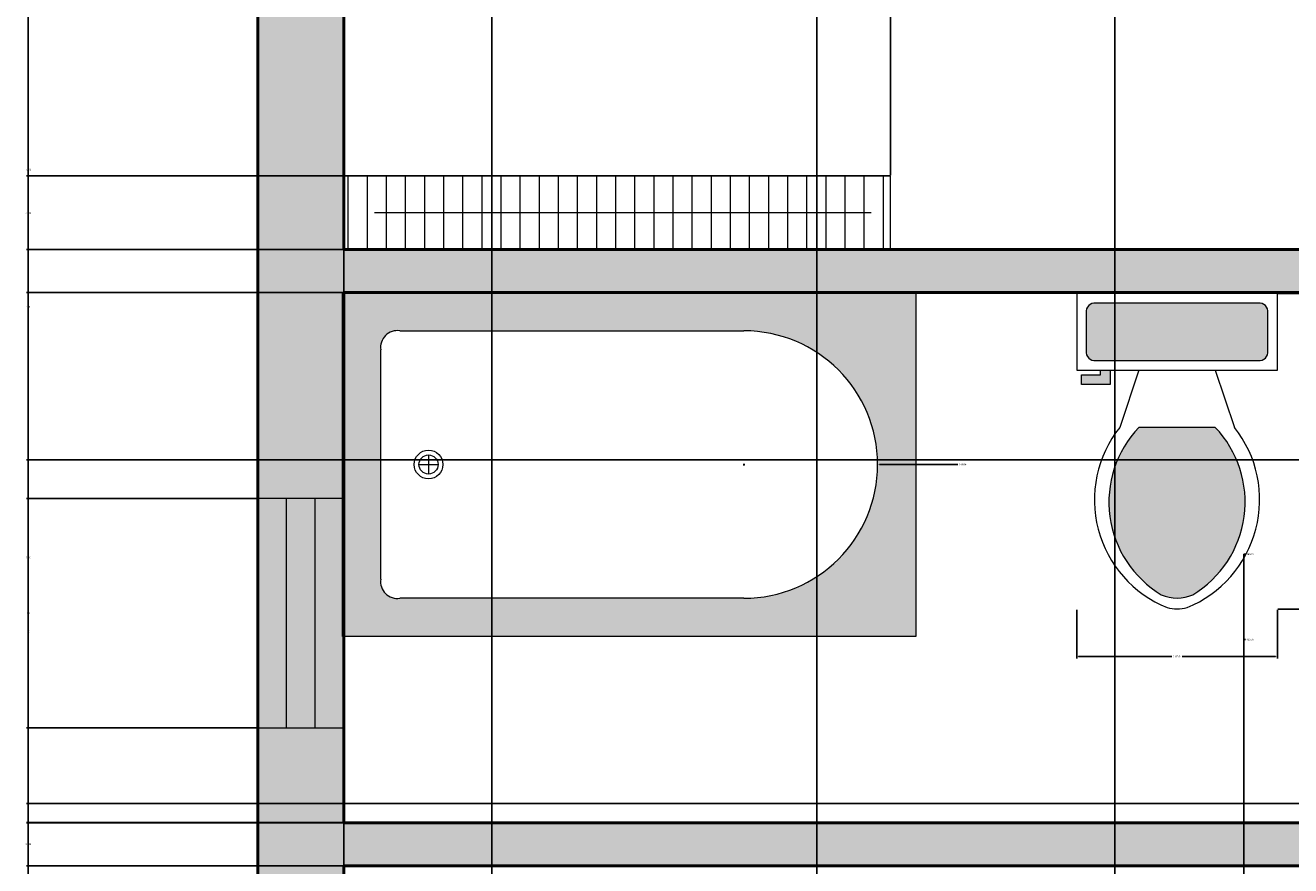
# Model space of a CAD drawing. Units: inches. Extents: x 1201 to 1754, y 247 to 775.
# Tile 6 of 10: x 1222 to 1355, y 557 to 645. Entities that reach past the tile are written whole.
import ezdxf

# ---------------------------------------------------------------- set-up
doc = ezdxf.new("R2010")
doc.units = ezdxf.units.IN
for name, color, linetype, lineweight in [('A-ANNO-DIMS', 2, 'Continuous', 18), ('A-FLOR-FIXT', 8, 'Continuous', 20), ('A-FLOR-PANL', 8, 'Continuous', 18), ('A-FLOR-PANL-PATT', 8, 'Continuous', 13), ('A-FURN-PATT', 9, 'Continuous', 13), ('A-GLAZ', 4, 'Continuous', 18), ('A-GLAZ-PATT', 9, 'Continuous', 13), ('A-WALL', 7, 'Continuous', 50), ('A-WALL-PATT', 9, 'Continuous', 13)]:
    doc.layers.add(name, color=color, linetype=linetype, lineweight=lineweight)
doc.styles.get("Standard").update_dxf_attribs({"font": 'arial.ttf'})
doc.dimstyles.get("Standard").update_dxf_attribs({"dimtxt": 0.18, "dimasz": 0.18, "dimexe": 0.18, "dimexo": 0.0625, "dimgap": 0.09, "dimtad": 0, "dimtih": 1, "dimtoh": 1, "dimdec": 4, "dimzin": 0, "dimdsep": 46, "dimtxsty": 'Standard', "dimcen": 0.09, "dimadec": 0, "dimazin": 0, "dimtfac": 1, "dimtdec": 4, "dimtofl": 0, "dimtmove": 0, "dimatfit": 3, "dimfxl": 1, "dimtolj": 1, "dimtzin": 0, "dimarcsym": 0})

# ---------------------------------------------------------------- blocks, each defined once
blk = doc.blocks.new('Bath Tub - 26 x 60 in.')
for p, q in [((9, -17), (9, -19)), ((8, -18), (10, -18))]:
    blk.add_line(p, q)
blk.add_lwpolyline([(0, -36), (0, 0), (60, 0), (60, -36)], close=True)
for points in [[(6, -4), (42, -4)], [(4, -30), (4, -6)], [(42, -32), (6, -32)]]:
    blk.add_lwpolyline(points)
for radius in [1.5, 1]:
    blk.add_circle((9, -18), radius)
for centre, radius, start, end in [((5.75, -5.75), 1.77, 81.8699, 188.1301), ((42, -18), 14, 270, 90), ((5.75, -30.25), 1.77, 171.8699, 278.1301)]:
    blk.add_arc(centre, radius, start, end)
blk = doc.blocks.new('Toilet - top')
for p, q in [((9.5, -6), (9.5, -2)), ((-10, -8.5), (-8, -8.5)), ((-10, -9.5), (-10, -8.5)), ((-8, -8.5), (-8, -8)), ((-7, -8), (-7, -9.5)), ((-4, -8), (-6, -14)), ((4, -8), (6, -14)), ((-7, -9.5), (-10, -9.5)), ((4, -14), (-4, -14))]:
    blk.add_line(p, q)
blk.add_lwpolyline([(10.5, -8), (10.5, 0), (-10.5, 0), (-10.5, -8)], close=True)
for points in [[(8.5, -1), (-8.5, -1)], [(-9.5, -2), (-9.5, -6)], [(-8.5, -7), (8.5, -7)]]:
    blk.add_lwpolyline(points)
for centre, radius, start, end in [((-8.62, -1.88), 0.884, 81.8699, 188.1301), ((8.62, -1.88), 0.884, 351.8699, 98.1301), ((-8.62, -6.12), 0.884, 171.8699, 278.1301), ((8.62, -6.12), 0.884, 261.8699, 8.1301), ((3.52, -21.58), 12.17, 141.4691, 247.9714), ((4.2, -21.82), 11.33, 136.3677, 238.9468), ((-3.52, -21.58), 12.17, 292.0284, 38.5307), ((-4.2, -21.82), 11.33, 301.053, 43.6321), ((0, -27.88), 4, 245.7318, 294.2682), ((0, -29), 4, 254.8605, 285.1395)]:
    blk.add_arc(centre, radius, start, end)
blk = doc.blocks.new('*D27')
at = {"layer": 'A-ANNO-DIMS', "color": 0, "lineweight": -2, "transparency": 16777216}
for p, q in [((1353.29, 617.33), (1358.37, 617.33)), ((1358.19, 617.15), (1358.19, 600.99)), ((1358.19, 584.47), (1358.19, 600.63)), ((1353.29, 584.29), (1358.37, 584.29))]:
    blk.add_line(p, q, dxfattribs=at)
at = {"layer": 'A-ANNO-DIMS', "color": 0, "transparency": 16777216}
for points in [[(1358.16, 617.15), (1358.22, 617.15), (1358.19, 617.33)], [(1358.16, 584.47), (1358.22, 584.47), (1358.19, 584.29)]]:
    blk.add_solid(points, dxfattribs=at)
at = {"layer": 'Defpoints', "color": 0, "transparency": 16777216}
for p in [(1353.23, 617.33), (1358.19, 617.33), (1353.23, 584.29)]:
    blk.add_point(p, dxfattribs=at)
at = {"layer": 'A-ANNO-DIMS', "color": 0, "transparency": 16777216, "insert": (1358.19, 600.81), "char_height": 0.18, "attachment_point": 5}
blk.add_mtext('\\A1;WC 33 TYP.', dxfattribs=at)
blk = doc.blocks.new('*D28')
at = {"layer": 'A-ANNO-DIMS', "color": 0, "lineweight": -2, "transparency": 16777216}
for p, q in [((1332.23, 584.22), (1332.23, 579.15)), ((1353.23, 584.22), (1353.23, 579.15)), ((1332.41, 579.33), (1342.2, 579.33)), ((1353.05, 579.33), (1343.26, 579.33))]:
    blk.add_line(p, q, dxfattribs=at)
at = {"layer": 'A-ANNO-DIMS', "color": 0, "transparency": 16777216}
for points in [[(1332.41, 579.36), (1332.41, 579.3), (1332.23, 579.33)], [(1353.05, 579.36), (1353.05, 579.3), (1353.23, 579.33)]]:
    blk.add_solid(points, dxfattribs=at)
at = {"layer": 'Defpoints', "color": 0, "transparency": 16777216}
for p in [(1332.23, 584.29), (1353.23, 584.29), (1353.23, 579.33)]:
    blk.add_point(p, dxfattribs=at)
at = {"layer": 'A-ANNO-DIMS', "color": 0, "transparency": 16777216, "insert": (1342.73, 579.33), "char_height": 0.18, "attachment_point": 5}
blk.add_mtext('\\A1;21 TYP.', dxfattribs=at)
blk = doc.blocks.new('*D48')
at = {"layer": 'A-ANNO-DIMS', "color": 0, "lineweight": -2, "transparency": 16777216}
for p, q in [((1255.46, 741.94), (1222.33, 741.94)), ((1222.51, 741.76), (1222.51, 682.12)), ((1222.51, 622.12), (1222.51, 681.76)), ((1255.46, 621.94), (1222.33, 621.94))]:
    blk.add_line(p, q, dxfattribs=at)
at = {"layer": 'A-ANNO-DIMS', "color": 0, "transparency": 16777216}
for points in [[(1222.48, 741.76), (1222.54, 741.76), (1222.51, 741.94)], [(1222.48, 622.12), (1222.54, 622.12), (1222.51, 621.94)]]:
    blk.add_solid(points, dxfattribs=at)
at = {"layer": 'Defpoints', "color": 0, "transparency": 16777216}
for p in [(1222.51, 741.94), (1255.52, 741.94), (1255.52, 621.94)]:
    blk.add_point(p, dxfattribs=at)
at = {"layer": 'A-ANNO-DIMS', "color": 0, "transparency": 16777216, "insert": (1222.51, 681.94), "char_height": 0.18, "attachment_point": 5}
blk.add_mtext('\\A1;120', dxfattribs=at)
blk = doc.blocks.new('*D49')
at = {"layer": 'A-ANNO-DIMS', "color": 0, "lineweight": -2, "transparency": 16777216}
for p, q in [((1394.96, 617.44), (1222.33, 617.44)), ((1222.51, 617.26), (1222.51, 589.87)), ((1222.51, 562.12), (1222.51, 589.51)), ((1394.96, 561.94), (1222.33, 561.94))]:
    blk.add_line(p, q, dxfattribs=at)
at = {"layer": 'A-ANNO-DIMS', "color": 0, "transparency": 16777216}
for points in [[(1222.48, 617.26), (1222.54, 617.26), (1222.51, 617.44)], [(1222.48, 562.12), (1222.54, 562.12), (1222.51, 561.94)]]:
    blk.add_solid(points, dxfattribs=at)
at = {"layer": 'Defpoints', "color": 0, "transparency": 16777216}
for p in [(1222.51, 617.44), (1395.02, 617.44), (1395.02, 561.94)]:
    blk.add_point(p, dxfattribs=at)
at = {"layer": 'A-ANNO-DIMS', "color": 0, "transparency": 16777216, "insert": (1222.51, 589.69), "char_height": 0.18, "attachment_point": 5}
blk.add_mtext('\\A1;55.5', dxfattribs=at)
blk = doc.blocks.new('*D52')
at = {"layer": 'A-ANNO-DIMS', "color": 0, "lineweight": -2, "transparency": 16777216}
for p, q in [((1477.46, 669.94), (1222.33, 669.94)), ((1222.51, 669.76), (1222.51, 616.12)), ((1222.51, 562.12), (1222.51, 615.76)), ((1477.46, 561.94), (1222.33, 561.94))]:
    blk.add_line(p, q, dxfattribs=at)
at = {"layer": 'A-ANNO-DIMS', "color": 0, "transparency": 16777216}
for points in [[(1222.48, 669.76), (1222.54, 669.76), (1222.51, 669.94)], [(1222.48, 562.12), (1222.54, 562.12), (1222.51, 561.94)]]:
    blk.add_solid(points, dxfattribs=at)
at = {"layer": 'Defpoints', "color": 0, "transparency": 16777216}
for p in [(1222.51, 669.94), (1477.52, 669.94), (1477.52, 561.94)]:
    blk.add_point(p, dxfattribs=at)
at = {"layer": 'A-ANNO-DIMS', "color": 0, "transparency": 16777216, "insert": (1222.51, 615.94), "char_height": 0.18, "attachment_point": 5}
blk.add_mtext('\\A1;108', dxfattribs=at)
blk = doc.blocks.new('*D54')
at = {"layer": 'A-ANNO-DIMS', "color": 0, "lineweight": -2, "transparency": 16777216}
for p, q in [((1255.52, 562), (1255.52, 775.14)), ((1255.7, 774.96), (1324.88, 774.96)), ((1394.84, 774.96), (1325.66, 774.96)), ((1395.02, 562), (1395.02, 775.14))]:
    blk.add_line(p, q, dxfattribs=at)
at = {"layer": 'A-ANNO-DIMS', "color": 0, "transparency": 16777216}
for points in [[(1255.7, 774.99), (1255.7, 774.93), (1255.52, 774.96)], [(1394.84, 774.99), (1394.84, 774.93), (1395.02, 774.96)]]:
    blk.add_solid(points, dxfattribs=at)
at = {"layer": 'Defpoints', "color": 0, "transparency": 16777216}
for p in [(1395.02, 774.96), (1255.52, 561.94), (1395.02, 561.94)]:
    blk.add_point(p, dxfattribs=at)
at = {"layer": 'A-ANNO-DIMS', "color": 0, "transparency": 16777216, "insert": (1325.27, 774.96), "char_height": 0.18, "attachment_point": 5}
blk.add_mtext('\\A1;139.5', dxfattribs=at)
blk = doc.blocks.new('*D59')
at = {"layer": 'A-ANNO-DIMS', "color": 0, "lineweight": -2, "transparency": 16777216}
for p, q in [((1255.52, 418), (1255.52, 775.14)), ((1255.7, 774.96), (1330.24, 774.96)), ((1405.34, 774.96), (1330.8, 774.96)), ((1405.52, 418), (1405.52, 775.14))]:
    blk.add_line(p, q, dxfattribs=at)
at = {"layer": 'A-ANNO-DIMS', "color": 0, "transparency": 16777216}
for points in [[(1255.7, 774.99), (1255.7, 774.93), (1255.52, 774.96)], [(1405.34, 774.99), (1405.34, 774.93), (1405.52, 774.96)]]:
    blk.add_solid(points, dxfattribs=at)
at = {"layer": 'Defpoints', "color": 0, "transparency": 16777216}
for p in [(1405.52, 774.96), (1255.52, 417.94), (1405.52, 417.94)]:
    blk.add_point(p, dxfattribs=at)
at = {"layer": 'A-ANNO-DIMS', "color": 0, "transparency": 16777216, "insert": (1330.52, 774.96), "char_height": 0.18, "attachment_point": 5}
blk.add_mtext('\\A1;150', dxfattribs=at)
blk = doc.blocks.new('*D65')
at = {"layer": 'A-ANNO-DIMS', "color": 0, "lineweight": -2, "transparency": 16777216}
for p, q in [((1471.46, 599.94), (1222.33, 599.94)), ((1222.51, 599.76), (1222.51, 582.12)), ((1222.51, 564.12), (1222.51, 581.76)), ((1471.46, 563.94), (1222.33, 563.94))]:
    blk.add_line(p, q, dxfattribs=at)
at = {"layer": 'A-ANNO-DIMS', "color": 0, "transparency": 16777216}
for points in [[(1222.48, 599.76), (1222.54, 599.76), (1222.51, 599.94)], [(1222.48, 564.12), (1222.54, 564.12), (1222.51, 563.94)]]:
    blk.add_solid(points, dxfattribs=at)
at = {"layer": 'Defpoints', "color": 0, "transparency": 16777216}
for p in [(1222.51, 599.94), (1471.52, 599.94), (1471.52, 563.94)]:
    blk.add_point(p, dxfattribs=at)
at = {"layer": 'A-ANNO-DIMS', "color": 0, "transparency": 16777216, "insert": (1222.51, 581.94), "char_height": 0.18, "attachment_point": 5}
blk.add_mtext('\\A1;36', dxfattribs=at)
blk = doc.blocks.new('*D71')
at = {"layer": 'A-ANNO-DIMS', "color": 0, "lineweight": -2, "transparency": 16777216}
for p, q in [((1246.46, 571.89), (1222.33, 571.89)), ((1222.51, 571.71), (1222.51, 539.47)), ((1222.51, 506.88), (1222.51, 539.11)), ((1246.46, 506.7), (1222.33, 506.7))]:
    blk.add_line(p, q, dxfattribs=at)
at = {"layer": 'A-ANNO-DIMS', "color": 0, "transparency": 16777216}
for points in [[(1222.48, 571.71), (1222.54, 571.71), (1222.51, 571.89)], [(1222.48, 506.88), (1222.54, 506.88), (1222.51, 506.7)]]:
    blk.add_solid(points, dxfattribs=at)
at = {"layer": 'Defpoints', "color": 0, "transparency": 16777216}
for p in [(1222.51, 571.89), (1246.52, 571.89), (1246.52, 506.7)]:
    blk.add_point(p, dxfattribs=at)
at = {"layer": 'A-ANNO-DIMS', "color": 0, "transparency": 16777216, "insert": (1222.51, 539.29), "char_height": 0.18, "attachment_point": 5}
blk.add_mtext('\\A1;65.19', dxfattribs=at)
blk = doc.blocks.new('*D72')
at = {"layer": 'A-ANNO-DIMS', "color": 0, "lineweight": -2, "transparency": 16777216}
for p, q in [((1246.46, 595.89), (1222.33, 595.89)), ((1222.51, 595.71), (1222.51, 584.07)), ((1222.51, 572.07), (1222.51, 583.71)), ((1246.46, 571.89), (1222.33, 571.89))]:
    blk.add_line(p, q, dxfattribs=at)
at = {"layer": 'A-ANNO-DIMS', "color": 0, "transparency": 16777216}
for points in [[(1222.48, 595.71), (1222.54, 595.71), (1222.51, 595.89)], [(1222.48, 572.07), (1222.54, 572.07), (1222.51, 571.89)]]:
    blk.add_solid(points, dxfattribs=at)
at = {"layer": 'Defpoints', "color": 0, "transparency": 16777216}
for p in [(1222.51, 595.89), (1246.52, 595.89), (1246.52, 571.89)]:
    blk.add_point(p, dxfattribs=at)
at = {"layer": 'A-ANNO-DIMS', "color": 0, "transparency": 16777216, "insert": (1222.51, 583.89), "char_height": 0.18, "attachment_point": 5}
blk.add_mtext('\\A1;24', dxfattribs=at)
blk = doc.blocks.new('*D73')
at = {"layer": 'A-ANNO-DIMS', "color": 0, "lineweight": -2, "transparency": 16777216}
for p, q in [((1246.46, 664.8), (1222.33, 664.8)), ((1222.51, 664.62), (1222.51, 630.52)), ((1222.51, 596.07), (1222.51, 630.16)), ((1246.46, 595.89), (1222.33, 595.89))]:
    blk.add_line(p, q, dxfattribs=at)
at = {"layer": 'A-ANNO-DIMS', "color": 0, "transparency": 16777216}
for points in [[(1222.48, 664.62), (1222.54, 664.62), (1222.51, 664.8)], [(1222.48, 596.07), (1222.54, 596.07), (1222.51, 595.89)]]:
    blk.add_solid(points, dxfattribs=at)
at = {"layer": 'Defpoints', "color": 0, "transparency": 16777216}
for p in [(1222.51, 664.8), (1246.52, 664.8), (1246.52, 595.89)]:
    blk.add_point(p, dxfattribs=at)
at = {"layer": 'A-ANNO-DIMS', "color": 0, "transparency": 16777216, "insert": (1222.51, 630.34), "char_height": 0.18, "attachment_point": 5}
blk.add_mtext('\\A1;68.91', dxfattribs=at)
blk = doc.blocks.new('*D83')
at = {"layer": 'A-ANNO-DIMS', "color": 0, "lineweight": -2, "transparency": 16777216}
for p, q in [((1471.46, 561.97), (1222.33, 561.97)), ((1222.51, 561.79), (1222.51, 559.89)), ((1222.51, 557.62), (1222.51, 559.52)), ((1471.46, 557.44), (1222.33, 557.44))]:
    blk.add_line(p, q, dxfattribs=at)
at = {"layer": 'A-ANNO-DIMS', "color": 0, "transparency": 16777216}
for points in [[(1222.48, 561.79), (1222.54, 561.79), (1222.51, 561.97)], [(1222.48, 557.62), (1222.54, 557.62), (1222.51, 557.44)]]:
    blk.add_solid(points, dxfattribs=at)
at = {"layer": 'Defpoints', "color": 0, "transparency": 16777216}
for p in [(1222.51, 561.97), (1471.52, 561.97), (1471.52, 557.44)]:
    blk.add_point(p, dxfattribs=at)
at = {"layer": 'A-ANNO-DIMS', "color": 0, "transparency": 16777216, "insert": (1222.51, 559.71), "char_height": 0.18, "attachment_point": 5}
blk.add_mtext('\\A1;4.528', dxfattribs=at)
blk = doc.blocks.new('*D85')
at = {"layer": 'A-ANNO-DIMS', "color": 0, "lineweight": -2, "transparency": 16777216}
for p, q in [((1255.52, 629.73), (1255.52, 775.14)), ((1255.7, 774.96), (1283.75, 774.96)), ((1312.55, 774.96), (1284.5, 774.96)), ((1312.73, 629.73), (1312.73, 775.14))]:
    blk.add_line(p, q, dxfattribs=at)
at = {"layer": 'A-ANNO-DIMS', "color": 0, "transparency": 16777216}
for points in [[(1255.7, 774.99), (1255.7, 774.93), (1255.52, 774.96)], [(1312.55, 774.99), (1312.55, 774.93), (1312.73, 774.96)]]:
    blk.add_solid(points, dxfattribs=at)
at = {"layer": 'Defpoints', "color": 0, "transparency": 16777216}
for p in [(1312.73, 774.96), (1255.52, 629.66), (1312.73, 629.66)]:
    blk.add_point(p, dxfattribs=at)
at = {"layer": 'A-ANNO-DIMS', "color": 0, "transparency": 16777216, "insert": (1284.13, 774.96), "char_height": 0.18, "attachment_point": 5}
blk.add_mtext('\\A1;57.21', dxfattribs=at)
blk = doc.blocks.new('*D86')
at = {"layer": 'A-ANNO-DIMS', "color": 0, "lineweight": -2, "transparency": 16777216}
for p, q in [((1312.67, 629.66), (1222.33, 629.66)), ((1222.51, 629.48), (1222.51, 625.98)), ((1222.51, 622.12), (1222.51, 625.62)), ((1312.67, 621.94), (1222.33, 621.94))]:
    blk.add_line(p, q, dxfattribs=at)
at = {"layer": 'A-ANNO-DIMS', "color": 0, "transparency": 16777216}
for points in [[(1222.48, 629.48), (1222.54, 629.48), (1222.51, 629.66)], [(1222.48, 622.12), (1222.54, 622.12), (1222.51, 621.94)]]:
    blk.add_solid(points, dxfattribs=at)
at = {"layer": 'Defpoints', "color": 0, "transparency": 16777216}
for p in [(1222.51, 629.66), (1312.73, 629.66), (1312.73, 621.94)]:
    blk.add_point(p, dxfattribs=at)
at = {"layer": 'A-ANNO-DIMS', "color": 0, "transparency": 16777216, "insert": (1222.51, 625.8), "char_height": 0.18, "attachment_point": 5}
blk.add_mtext('\\A1;7.721', dxfattribs=at)
blk = doc.blocks.new('*D94')
at = {"layer": 'A-ANNO-DIMS', "color": 0, "lineweight": -2, "transparency": 16777216}
for p, q in [((1305.02, 443.29), (1305.02, 775.14)), ((1305.2, 774.96), (1320.15, 774.96)), ((1336.03, 774.96), (1321.08, 774.96)), ((1336.21, 449.65), (1336.21, 775.14))]:
    blk.add_line(p, q, dxfattribs=at)
at = {"layer": 'A-ANNO-DIMS', "color": 0, "transparency": 16777216}
for points in [[(1305.2, 774.99), (1305.2, 774.93), (1305.02, 774.96)], [(1336.03, 774.99), (1336.03, 774.93), (1336.21, 774.96)]]:
    blk.add_solid(points, dxfattribs=at)
at = {"layer": 'Defpoints', "color": 0, "transparency": 16777216}
for p in [(1336.21, 774.96), (1336.21, 449.58), (1305.02, 443.23)]:
    blk.add_point(p, dxfattribs=at)
at = {"layer": 'A-ANNO-DIMS', "color": 0, "transparency": 16777216, "insert": (1320.61, 774.96), "char_height": 0.18, "attachment_point": 5}
blk.add_mtext('\\A1;31.195', dxfattribs=at)
blk = doc.blocks.new('*D97')
at = {"layer": 'A-ANNO-DIMS', "color": 0, "lineweight": -2, "transparency": 16777216}
for p, q in [((1255.52, 506.76), (1255.52, 775.14)), ((1255.7, 774.96), (1262.81, 774.96)), ((1270.84, 774.96), (1263.72, 774.96)), ((1271.02, 485.29), (1271.02, 775.14))]:
    blk.add_line(p, q, dxfattribs=at)
at = {"layer": 'A-ANNO-DIMS', "color": 0, "transparency": 16777216}
for points in [[(1255.7, 774.99), (1255.7, 774.93), (1255.52, 774.96)], [(1270.84, 774.99), (1270.84, 774.93), (1271.02, 774.96)]]:
    blk.add_solid(points, dxfattribs=at)
at = {"layer": 'Defpoints', "color": 0, "transparency": 16777216}
for p in [(1271.02, 774.96), (1255.52, 506.7), (1271.02, 485.23)]:
    blk.add_point(p, dxfattribs=at)
at = {"layer": 'A-ANNO-DIMS', "color": 0, "transparency": 16777216, "insert": (1263.27, 774.96), "char_height": 0.18, "attachment_point": 5}
blk.add_mtext('\\A1;15.496', dxfattribs=at)
blk = doc.blocks.new('*D103')
at = {"layer": 'A-ANNO-DIMS', "color": 0, "lineweight": -2, "transparency": 16777216}
for p, q in [((1349.89, 590.05), (1349.71, 590.05)), ((1349.71, 590.05), (1349.71, 554.08)), ((1349.62, 493.65), (1349.8, 493.65)), ((1349.71, 493.56), (1349.71, 493.74))]:
    blk.add_line(p, q, dxfattribs=at)
at = {"layer": 'A-ANNO-DIMS', "color": 0, "transparency": 16777216}
blk.add_solid([(1349.68, 554.08), (1349.74, 554.08), (1349.71, 553.9)], dxfattribs=at)
at = {"layer": 'Defpoints', "color": 0, "transparency": 16777216}
for p in [(1349.71, 553.9), (1349.71, 493.65)]:
    blk.add_point(p, dxfattribs=at)
at = {"layer": 'A-ANNO-DIMS', "color": 0, "transparency": 16777216, "insert": (1350.37, 590.05), "char_height": 0.18, "attachment_point": 5}
blk.add_mtext('\\A1;R60.25', dxfattribs=at)
blk = doc.blocks.new('*D104')
at = {"layer": 'A-ANNO-DIMS', "color": 0, "lineweight": -2, "transparency": 16777216}
for p, q in [((1349.89, 581.13), (1349.71, 581.13)), ((1349.71, 581.13), (1349.71, 548.08)), ((1349.62, 492.52), (1349.8, 492.52)), ((1349.71, 492.43), (1349.71, 492.61))]:
    blk.add_line(p, q, dxfattribs=at)
at = {"layer": 'A-ANNO-DIMS', "color": 0, "transparency": 16777216}
blk.add_solid([(1349.68, 548.08), (1349.74, 548.08), (1349.71, 547.9)], dxfattribs=at)
at = {"layer": 'Defpoints', "color": 0, "transparency": 16777216}
for p in [(1349.71, 547.9), (1349.71, 492.52)]:
    blk.add_point(p, dxfattribs=at)
at = {"layer": 'A-ANNO-DIMS', "color": 0, "transparency": 16777216, "insert": (1350.37, 581.13), "char_height": 0.18, "attachment_point": 5}
blk.add_mtext('\\A1;R55.38', dxfattribs=at)
blk = doc.blocks.new('*D105')
at = {"layer": 'A-ANNO-DIMS', "color": 0, "lineweight": -2, "transparency": 16777216}
for p, q in [((1297.31, 599.44), (1297.49, 599.44)), ((1297.4, 599.35), (1297.4, 599.53)), ((1319.8, 599.44), (1311.58, 599.44))]:
    blk.add_line(p, q, dxfattribs=at)
at = {"layer": 'A-ANNO-DIMS', "color": 0, "transparency": 16777216}
blk.add_solid([(1311.58, 599.47), (1311.58, 599.41), (1311.4, 599.44)], dxfattribs=at)
at = {"layer": 'Defpoints', "color": 0, "transparency": 16777216}
for p in [(1297.4, 599.44), (1311.4, 599.44)]:
    blk.add_point(p, dxfattribs=at)
at = {"layer": 'A-ANNO-DIMS', "color": 0, "transparency": 16777216, "insert": (1320.3, 599.44), "char_height": 0.18, "attachment_point": 5}
blk.add_mtext('\\A1;2X R14', dxfattribs=at)

msp = doc.modelspace()

# ---------------------------------------------------------------- hatches: boundary and pattern name
at = {"layer": 'A-FLOR-PANL-PATT'}
h = msp.add_hatch(dxfattribs=at)
h.set_pattern_fill('ANSI31', color=256, scale=0.629921, angle=45, style=0)
h.paths.add_polyline_path([(1255.5208, 621.9415), (1312.7334, 621.9415), (1312.7334, 629.6628), (1255.5208, 629.6628)])
at = {"layer": 'A-FURN-PATT'}
h = msp.add_hatch(color=256, dxfattribs=at)
h.dxf.hatch_style = 1
h.paths.add_polyline_path([(1335.0621, 716.0469), (1322.6678, 716.0469), (1322.6678, 726.4842), (1286.1373, 726.4842), (1286.1373, 674.95), (1335.0621, 674.95)])
h.paths.add_polyline_path([(1328.5388, 739.2047), (1311.5782, 739.2047), (1311.5782, 728.4412), (1322.6678, 728.4412), (1324.2987, 726.8104), (1328.5388, 726.8104)])
h.paths.add_polyline_path([(1309.6212, 739.2047), (1292.6606, 739.2047), (1292.6606, 728.4412), (1309.6212, 728.4412)])
h.paths.add_polyline_path([(1346.7317, 603.3316), (1338.7317, 603.3316, 0.48007965), (1341.0876, 585.8086, 0.21500378), (1344.3757, 585.8086, 0.4800795)])
h.paths.add_polyline_path([(1315.398, 617.4415), (1255.5208, 617.4415), (1255.5208, 581.4415), (1315.398, 581.4415)])
h.paths.add_polyline_path([(1297.398, 585.4415), (1261.398, 585.4415, -0.50000012), (1259.398, 587.4415), (1259.398, 611.4415, -0.50000012), (1261.398, 613.4415), (1297.398, 613.4415, -1)], flags=16)
h.paths.add_polyline_path([(1262.898, 599.4415, -1), (1265.898, 599.4415, -1)], flags=0)
h.paths.add_polyline_path([(1263.398, 599.4415, -1), (1265.398, 599.4415, -1)], flags=0)
h.paths.add_polyline_path([(1352.2316, 615.3316, 0.50000012), (1351.2316, 616.3316), (1334.2316, 616.3316, 0.50000012), (1333.2316, 615.3316), (1333.2316, 611.3316, 0.50000012), (1334.2316, 610.3316), (1351.2316, 610.3316, 0.50000012), (1352.2316, 611.3316)])
h.paths.add_polyline_path([(1335.7316, 609.3316), (1334.7316, 609.3316), (1334.7316, 608.8316), (1332.7316, 608.8316), (1332.7316, 607.8316), (1335.7316, 607.8316)])
h.paths.add_polyline_path([(1537.5652, 741.6115), (1477.5652, 741.6115), (1477.5652, 705.6115), (1537.5652, 705.6115)])
h.paths.add_polyline_path([(1519.5652, 709.6115), (1483.5652, 709.6115, -0.50000012), (1481.5652, 711.6115), (1481.5652, 735.6115, -0.50000012), (1483.5652, 737.6115), (1519.5652, 737.6115, -1)], flags=16)
h.paths.add_polyline_path([(1485.0652, 723.6115, -1), (1488.0652, 723.6115, -1)], flags=0)
h.paths.add_polyline_path([(1485.5652, 723.6115, -1), (1487.5652, 723.6115, -1)], flags=0)
h.paths.add_polyline_path([(1712.1885, 727.9922), (1704.1885, 727.9922, 0.48007965), (1706.5444, 710.4693, 0.21500378), (1709.8325, 710.4693, 0.4800795)])
h.paths.add_polyline_path([(1701.1884, 733.9922), (1700.1884, 733.9922), (1700.1884, 733.4922), (1698.1884, 733.4922), (1698.1884, 732.4922), (1701.1884, 732.4922)])
h.paths.add_polyline_path([(1717.5208, 740.6473, 0.27397494), (1716.6884, 740.9922), (1699.6884, 740.9922, 0.50000012), (1698.6884, 739.9922), (1698.6884, 735.9922, 0.50000012), (1699.6884, 734.9922), (1716.6884, 734.9922, 0.27397494), (1717.5208, 735.3372)])
h.paths.add_polyline_path([(1586.346, 642.6772), (1573.9517, 642.6772), (1573.9517, 653.1145), (1537.4212, 653.1145), (1537.4212, 601.5803), (1586.346, 601.5803)])
h.paths.add_polyline_path([(1579.8227, 665.835), (1562.8621, 665.835), (1562.8621, 655.0715), (1573.9517, 655.0715), (1575.5826, 653.4407), (1579.8227, 653.4407)])
h.paths.add_polyline_path([(1560.9051, 665.835), (1543.9445, 665.835), (1543.9445, 655.0715), (1560.9051, 655.0715)])
at = {"layer": 'A-GLAZ-PATT'}
h = msp.add_hatch(color=256, dxfattribs=at)
h.dxf.hatch_style = 1
h.set_gradient(color1=(0, 0, 255), color2=(255, 255, 0), name='INVSPHERICAL')
h.paths.add_polyline_path([(1249.5208, 595.8878), (1246.5208, 595.8878), (1246.5208, 571.8878), (1249.5208, 571.8878)])
h.paths.add_polyline_path([(1252.5208, 595.8878), (1249.5208, 595.8878), (1249.5208, 571.8878), (1252.5208, 571.8878)])
h.paths.add_polyline_path([(1255.398, 595.8878), (1252.5208, 595.8878), (1252.5208, 571.8878), (1255.5208, 571.8878), (1255.5208, 581.4415), (1255.398, 581.4415)])
at = {"layer": 'A-WALL-PATT'}
h = msp.add_hatch(color=256, dxfattribs=at)
h.dxf.hatch_style = 1
h.paths.add_polyline_path([(1255.5208, 741.9415), (1471.5208, 741.9415), (1471.5208, 684.2327), (1471.5208, 602.9415), (1477.5208, 602.9415), (1477.5208, 669.9415), (1618.5208, 669.9415), (1618.5208, 674.4415), (1477.5208, 674.4415), (1477.5208, 741.9415), (1481.2969, 741.9415), (1481.2969, 750.9415), (1246.5208, 750.9415), (1246.5208, 700.7954), (1255.5208, 700.7954)])
h.paths.add_polyline_path([(1255.5208, 557.4415), (1399.5208, 557.4415), (1399.5208, 617.4415), (1423.5208, 617.4415), (1423.5208, 621.9415), (1392.0208, 621.9415), (1392.0208, 617.4415), (1395.0208, 617.4415), (1395.0208, 561.9415), (1255.5208, 561.9415), (1255.5208, 571.8878), (1246.5208, 571.8878), (1246.5208, 506.6967), (1255.5208, 506.6967)])
h.paths.add_polyline_path([(1255.5208, 664.7954), (1246.5208, 664.7954), (1246.5208, 595.8878), (1255.398, 595.8878), (1255.398, 617.4415), (1315.398, 617.4415), (1356.0208, 617.4415), (1356.0208, 618.0127), (1356.0208, 621.9415), (1255.5208, 621.9415), (1255.5208, 629.6628)])
h.paths.add_polyline_path([(1255.5208, 470.6967), (1246.5208, 470.6967), (1246.5208, 347.7487), (1255.5208, 347.7487), (1255.5208, 413.4415), (1405.5208, 413.4415), (1405.5208, 417.9415), (1255.5208, 417.9415)])
h.paths.add_polyline_path([(1290.9481, 279.9415), (1255.5208, 279.9415), (1255.5208, 311.7487), (1246.5208, 311.7487), (1246.5208, 270.9415), (1290.9481, 270.9415)])
h.paths.add_polyline_path([(1486.5907, 279.9415), (1477.5208, 279.9415), (1477.5208, 417.9415), (1468.5208, 417.9415), (1468.5208, 413.4415), (1471.5208, 413.4415), (1471.5208, 279.9415), (1399.0105, 279.9415), (1399.0105, 270.9415), (1486.5907, 270.9415)])
h.paths.add_polyline_path([(1563.0208, 279.9415), (1542.0208, 279.9415), (1542.0208, 417.9415), (1501.5208, 417.9415), (1501.5208, 413.4415), (1513.81, 413.4415), (1513.8125, 413.6987), (1537.8114, 413.4623), (1537.5208, 383.9637), (1537.5208, 279.9415), (1522.5907, 279.9415), (1522.5907, 270.9415), (1563.0208, 270.9415)])
h.paths.add_polyline_path([(1726.5208, 404.0342), (1717.5208, 404.0342), (1717.5208, 279.9415), (1641.0208, 279.9415), (1641.0208, 270.9415), (1726.5208, 270.9415)])
h.paths.add_polyline_path([(1726.5208, 507.4363), (1717.5208, 507.4363), (1717.5208, 440.0342), (1726.5208, 440.0342)])
h.paths.add_polyline_path([(1726.5208, 611.6009), (1717.5208, 611.6009), (1717.5208, 561.9415), (1477.5208, 561.9415), (1471.5208, 561.9692), (1471.5208, 557.4415), (1717.5208, 557.4415), (1717.5208, 543.4363), (1726.5208, 543.4363)])
h.paths.add_polyline_path([(1726.5208, 750.9415), (1505.2969, 750.9415), (1505.2969, 741.9415), (1697.6884, 741.9415), (1697.6884, 741.9922), (1718.6884, 741.9922), (1718.6884, 733.9922), (1717.5208, 733.9922), (1717.5208, 674.4415), (1660.5208, 674.4415), (1660.5208, 669.9415), (1717.5208, 669.9415), (1717.5208, 647.6009), (1726.5208, 647.6009)])

# ---------------------------------------------------------------- linework, layer by layer
at = {"layer": 'A-FLOR-PANL'}
for p, q in [((1312.7334, 629.6628), (1255.5208, 629.6628)), ((1255.5208, 629.6628), (1255.5208, 621.9415)), ((1312.7334, 621.9415), (1312.7334, 629.6628)), ((1310.7334, 625.8021), (1258.7334, 625.8021)), ((1255.5208, 621.9415), (1312.7334, 621.9415))]:
    msp.add_line(p, q, dxfattribs=at)
at = {"layer": 'A-GLAZ'}
for p, q in [((1249.5208, 571.8878), (1249.5208, 595.8878)), ((1252.5208, 571.8878), (1252.5208, 595.8878))]:
    msp.add_line(p, q, dxfattribs=at)
msp.add_lwpolyline([(1246.5208, 595.8878), (1246.5208, 571.8878), (1255.5208, 571.8878), (1255.5208, 595.8878)], close=True, dxfattribs=at)
at = {"layer": 'A-WALL'}
for p, q in [((1255.5208, 741.9415), (1255.5208, 621.9415)), ((1356.0208, 621.9415), (1255.5208, 621.9415)), ((1356.0208, 617.4415), (1255.5208, 617.4415)), ((1255.5208, 617.4415), (1255.5208, 561.9415)), ((1395.0208, 561.9415), (1255.5208, 561.9415)), ((1399.5208, 557.4415), (1255.5208, 557.4415)), ((1255.5208, 557.4415), (1255.5208, 417.9415))]:
    msp.add_line(p, q, dxfattribs=at)
msp.add_lwpolyline([(1638.0208, 270.9415), (1726.5208, 270.9415), (1726.5208, 750.9415), (1246.5208, 750.9415), (1246.5208, 270.9415), (1566.0208, 270.9415)], dxfattribs=at)

# ---------------------------------------------------------------- block references
at = {"layer": 'A-FLOR-FIXT'}
for name, p in [('Bath Tub - 26 x 60 in.', (1255.398, 617.4415)), ('Toilet - top', (1342.7316, 617.3316))]:
    msp.add_blockref(name, p, dxfattribs=at)

# ---------------------------------------------------------------- dimensions: what is measured, and where the dimension line sits
at = {"layer": 'A-ANNO-DIMS'}
for base, p1, p2, override, picture, middle in [((1395.0208, 774.9565), (1255.5208, 561.9415), (1395.0208, 561.9415), {"dimdec": 1, "dimlfac": 1, "dimrnd": 0, "dimzin": 0, "dimdsep": 46, "dimlunit": 2}, '*D54', (1325.2708, 774.9565)), ((1405.5208, 774.9565), (1255.5208, 417.9415), (1405.5208, 417.9415), {"dimdec": 0, "dimlfac": 1, "dimrnd": 0, "dimzin": 0, "dimdsep": 46, "dimlunit": 2}, '*D59', (1330.5208, 774.9565)), ((1312.7334, 774.9565), (1255.5208, 629.6628), (1312.7334, 629.6628), {"dimdec": 2, "dimlfac": 1, "dimrnd": 0, "dimzin": 0, "dimdsep": 46, "dimlunit": 2}, '*D85', (1284.1271, 774.9565)), ((1271.0165, 774.9565), (1255.5208, 506.6967), (1271.0165, 485.2267), {"dimdec": 3, "dimlfac": 1, "dimrnd": 0, "dimzin": 0, "dimdsep": 46, "dimlunit": 2}, '*D97', (1263.2686, 774.9565)), ((1336.2113, 774.9565), (1305.0165, 443.2267), (1336.2113, 449.5839), {"dimdec": 3, "dimlfac": 1, "dimrnd": 0, "dimzin": 0, "dimdsep": 46, "dimlunit": 2}, '*D94', (1320.6139, 774.9565))]:
    dim = msp.add_linear_dim(base=base, p1=p1, p2=p2, dimstyle='Standard', override=override, dxfattribs=at)
    dim.commit()
    dim.dimension.update_dxf_attribs({"geometry": picture, "text_midpoint": middle})
for base, p1, p2, override, picture, middle in [((1222.5058, 741.9415), (1255.5208, 621.9415), (1255.5208, 741.9415), {"dimdec": 0, "dimlfac": 1, "dimrnd": 0, "dimzin": 0, "dimdsep": 46, "dimlunit": 2}, '*D48', (1222.5058, 681.9415)), ((1222.5058, 669.9415), (1477.5208, 561.9415), (1477.5208, 669.9415), {"dimdec": 0, "dimlfac": 1, "dimrnd": 0, "dimzin": 0, "dimdsep": 46, "dimlunit": 2}, '*D52', (1222.5058, 615.9415)), ((1222.5058, 664.7954), (1246.5208, 595.8878), (1246.5208, 664.7954), {"dimdec": 2, "dimlfac": 1, "dimrnd": 0, "dimzin": 0, "dimdsep": 46, "dimlunit": 2}, '*D73', (1222.5058, 630.3416)), ((1222.5058, 629.6628), (1312.7334, 621.9415), (1312.7334, 629.6628), {"dimdec": 3, "dimlfac": 1, "dimrnd": 0, "dimzin": 0, "dimdsep": 46, "dimlunit": 2}, '*D86', (1222.5058, 625.8021)), ((1222.5058, 617.4415), (1395.0208, 561.9415), (1395.0208, 617.4415), {"dimdec": 1, "dimlfac": 1, "dimrnd": 0, "dimzin": 0, "dimdsep": 46, "dimlunit": 2}, '*D49', (1222.5058, 589.6915)), ((1222.5058, 599.9415), (1471.5208, 563.9415), (1471.5208, 599.9415), {"dimdec": 0, "dimlfac": 1, "dimrnd": 0, "dimzin": 0, "dimdsep": 46, "dimlunit": 2}, '*D65', (1222.5058, 581.9415)), ((1222.5058, 595.8878), (1246.5208, 571.8878), (1246.5208, 595.8878), {"dimdec": 0, "dimlfac": 1, "dimrnd": 0, "dimzin": 0, "dimdsep": 46, "dimlunit": 2}, '*D72', (1222.5058, 583.8878)), ((1222.5058, 571.8878), (1246.5208, 506.6967), (1246.5208, 571.8878), {"dimdec": 2, "dimlfac": 1, "dimrnd": 0, "dimzin": 0, "dimdsep": 46, "dimlunit": 2}, '*D71', (1222.5058, 539.2922)), ((1222.5058, 561.9692), (1471.5208, 557.4415), (1471.5208, 561.9692), {"dimdec": 3, "dimlfac": 1, "dimrnd": 0, "dimzin": 0, "dimdsep": 46, "dimlunit": 2}, '*D83', (1222.5058, 559.7053))]:
    dim = msp.add_linear_dim(base=base, p1=p1, p2=p2, angle=90, dimstyle='Standard', override=override, dxfattribs=at)
    dim.commit()
    dim.dimension.update_dxf_attribs({"geometry": picture, "text_midpoint": middle})
dim = msp.add_linear_dim(base=(1358.1885, 617.3316), p1=(1353.2316, 584.2854), p2=(1353.2316, 617.3316), angle=90, text='WC <> TYP.', dimstyle='Standard', override={"dimdec": 0, "dimlfac": 1, "dimrnd": 0, "dimzin": 0, "dimdsep": 46, "dimlunit": 2}, dxfattribs=at)
dim.commit()
dim.dimension.update_dxf_attribs({"geometry": '*D27', "text_midpoint": (1358.1885, 600.8085)})
dim = msp.add_radius_dim(center=(1297.398, 599.4415), mpoint=(1311.398, 599.441), text='2X <>', dimstyle='Standard', override={"dimdec": 0, "dimlfac": 1, "dimrnd": 0, "dimzin": 0, "dimdsep": 46, "dimlunit": 2}, dxfattribs=at)
dim.commit()
dim.dimension.update_dxf_attribs({"geometry": '*D105', "text_midpoint": (1319.798, 599.4407), "dimtype": 164})
for center, mpoint, picture, middle in [((1349.7056, 493.6535), (1349.706, 553.9035), '*D103', (1350.3667, 590.0534)), ((1349.7056, 492.5191), (1349.706, 547.9035), '*D104', (1350.3662, 581.1342))]:
    dim = msp.add_radius_dim(center=center, mpoint=mpoint, dimstyle='Standard', override={"dimdec": 2, "dimlfac": 1, "dimrnd": 0, "dimzin": 0, "dimdsep": 46, "dimlunit": 2}, dxfattribs=at)
    dim.commit()
    dim.dimension.update_dxf_attribs({"geometry": picture, "text_midpoint": middle, "dimtype": 164})
dim = msp.add_linear_dim(base=(1353.2316, 579.3284), p1=(1332.2316, 584.2854), p2=(1353.2316, 584.2854), text='<> TYP.', dimstyle='Standard', override={"dimdec": 0, "dimlfac": 1, "dimrnd": 0, "dimzin": 0, "dimdsep": 46, "dimlunit": 2}, dxfattribs=at)
dim.commit()
dim.dimension.update_dxf_attribs({"geometry": '*D28', "text_midpoint": (1342.7316, 579.3284)})

doc.saveas('drawing.dxf')
